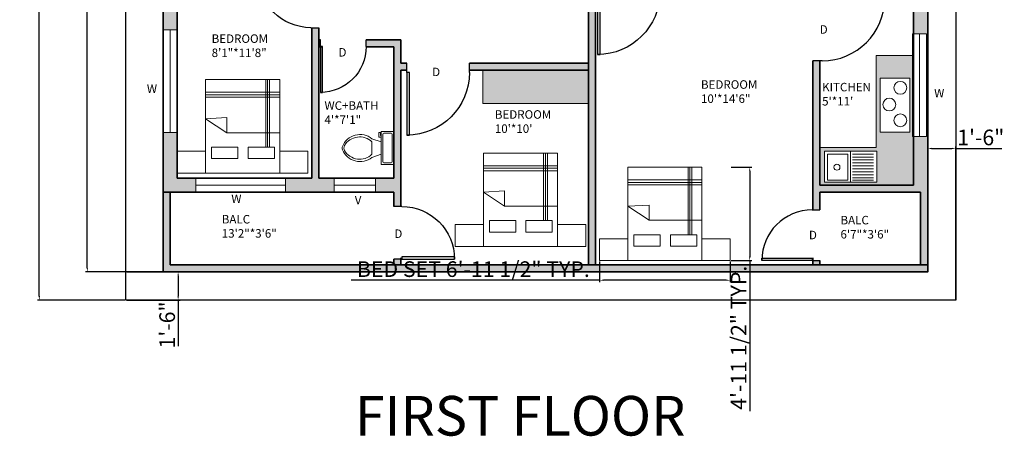
# Model space of a CAD drawing. Units: inches. Extents: x 2048 to 2702, y 2180 to 2964.
# Tile 1 of 3: x 2056 to 2686, y 2180 to 2447. Entities that reach past the tile are written whole.
import ezdxf

# ---------------------------------------------------------------- set-up
doc = ezdxf.new("R2010")
doc.units = ezdxf.units.IN
for name, color, linetype, lineweight in [('A-ANNO-DIMS', 2, 'Continuous', 13), ('A-ANNO-TEXT', 130, 'Continuous', 18), ('A-AREA-IDEN', 130, 'Continuous', 18), ('A-CASE-PATT', 142, 'Continuous', 13), ('A-DOOR', 4, 'Continuous', 25), ('A-EQPM', 142, 'Continuous', 18), ('A-FLOR-FIXT', 142, 'Continuous', 18), ('A-FURN-PATT', 191, 'Continuous', 13), ('A-GLAZ', 4, 'Continuous', 18), ('A-WALL-PATT', 174, 'Continuous', 13), ('bed', 62, 'Continuous', 18), ('C-PROP', 7, 'Continuous', 25), ('kit', 142, 'Continuous', 18), ('TOI', 210, 'Continuous', 18), ('wall', 174, 'Continuous', 35), ('ward', 191, 'Continuous', 18)]:
    doc.layers.add(name, color=color, linetype=linetype, lineweight=lineweight)
doc.styles.get("Standard").update_dxf_attribs({"font": 'arial.ttf'})
doc.dimstyles.new('ISO-25', dxfattribs={"dimtxt": 10, "dimasz": 2.5, "dimexe": 1.25, "dimexo": 0.625, "dimtad": 1, "dimdec": 0, "dimlunit": 4, "dimtxsty": 'Standard', "dimcen": 2.5, "dimadec": 0, "dimazin": 0, "dimtfac": 1, "dimtdec": 0, "dimtmove": 0, "dimatfit": 3, "dimfxl": 1, "dimarcsym": 0})

# ---------------------------------------------------------------- blocks, each defined once
blk = doc.blocks.new('*U2')
for p, q in [((0, 0), (0, -6)), ((40, 0), (40, -6))]:
    blk.add_line(p, q)
blk.add_lwpolyline([(0, 0), (0, 40), (1.75, 40), (1.75, 0)], close=True)
blk.add_arc((0, 0), 40, 0, 90)
blk = doc.blocks.new('*U4')
for p, q in [((9.5, -6), (9.5, -2)), ((-10, -8.5), (-8, -8.5)), ((-10, -9.5), (-10, -8.5)), ((-7, -9.5), (-10, -9.5)), ((-8, -8.5), (-8, -8)), ((-7, -8), (-7, -9.5)), ((-4, -8), (-6, -14)), ((4, -8), (6, -14)), ((4, -14), (-4, -14))]:
    blk.add_line(p, q)
blk.add_lwpolyline([(10.5, -8), (10.5, 0), (-10.5, 0), (-10.5, -8)], close=True)
for points in [[(-9.5, -2), (-9.5, -6)], [(8.5, -1), (-8.5, -1)], [(-8.5, -7), (8.5, -7)]]:
    blk.add_lwpolyline(points)
for centre, radius, start, end in [((-8.62, -1.88), 0.884, 81.8699, 188.1301), ((-8.62, -6.12), 0.884, 171.8699, 278.1301), ((8.62, -1.88), 0.884, 351.8699, 98.1301), ((8.62, -6.12), 0.884, 261.8699, 8.1301), ((3.52, -21.58), 12.17, 141.46911, 247.97143), ((4.2, -21.82), 11.33, 136.36773, 238.94682), ((-3.52, -21.58), 12.17, 292.02843, 38.53071), ((-4.2, -21.82), 11.33, 301.05301, 43.63209), ((0, -27.88), 4, 245.73182, 294.26817), ((0, -29), 4, 254.86053, 285.13947)]:
    blk.add_arc(centre, radius, start, end)
blk = doc.blocks.new('*D11')
at = {"layer": 'A-ANNO-DIMS', "color": 0, "lineweight": -2, "transparency": 16777216}
for p, q in [((2123.4, 2813.51), (2067.51, 2813.51)), ((2068.76, 2270.01), (2068.76, 2811.01)), ((2123.4, 2267.51), (2067.51, 2267.51))]:
    blk.add_line(p, q, dxfattribs=at)
at = {"layer": 'A-ANNO-DIMS', "color": 0, "transparency": 16777216}
for points in [[(2068.35, 2811.01), (2069.18, 2811.01), (2068.76, 2813.51)], [(2068.35, 2270.01), (2069.18, 2270.01), (2068.76, 2267.51)]]:
    blk.add_solid(points, dxfattribs=at)
at = {"layer": 'Defpoints', "color": 0, "transparency": 16777216}
for p in [(2068.76, 2813.51), (2124.03, 2813.51), (2124.03, 2267.51)]:
    blk.add_point(p, dxfattribs=at)
at = {"layer": 'A-ANNO-DIMS', "color": 0, "transparency": 16777216, "insert": (2063.03, 2540.51), "char_height": 10, "attachment_point": 5, "rotation": 90}
blk.add_mtext('45\'-6"', dxfattribs=at)
blk = doc.blocks.new('*D12')
at = {"layer": 'A-ANNO-DIMS', "color": 0, "lineweight": -2, "transparency": 16777216}
for p, q in [((2147.4, 2789.51), (2098.23, 2789.51)), ((2099.48, 2288.01), (2099.48, 2787.01)), ((2147.4, 2285.51), (2098.23, 2285.51))]:
    blk.add_line(p, q, dxfattribs=at)
at = {"layer": 'A-ANNO-DIMS', "color": 0, "transparency": 16777216}
for points in [[(2099.06, 2787.01), (2099.89, 2787.01), (2099.48, 2789.51)], [(2099.06, 2288.01), (2099.89, 2288.01), (2099.48, 2285.51)]]:
    blk.add_solid(points, dxfattribs=at)
at = {"layer": 'Defpoints', "color": 0, "transparency": 16777216}
for p in [(2099.48, 2789.51), (2148.03, 2789.51), (2148.03, 2285.51)]:
    blk.add_point(p, dxfattribs=at)
at = {"layer": 'A-ANNO-DIMS', "color": 0, "transparency": 16777216, "insert": (2093.83, 2537.51), "char_height": 10, "attachment_point": 5, "rotation": 90}
blk.add_mtext("42'", dxfattribs=at)
blk = doc.blocks.new('*D13')
at = {"layer": 'A-ANNO-DIMS', "color": 0, "lineweight": -2, "transparency": 16777216}
for p, q in [((2124.65, 2285.51), (2158.82, 2285.51)), ((2157.57, 2283.01), (2157.57, 2270.01)), ((2124.65, 2267.51), (2158.82, 2267.51)), ((2157.57, 2267.51), (2157.57, 2238.12))]:
    blk.add_line(p, q, dxfattribs=at)
at = {"layer": 'A-ANNO-DIMS', "color": 0, "transparency": 16777216}
for points in [[(2157.15, 2283.01), (2157.99, 2283.01), (2157.57, 2285.51)], [(2157.15, 2270.01), (2157.99, 2270.01), (2157.57, 2267.51)]]:
    blk.add_solid(points, dxfattribs=at)
at = {"layer": 'Defpoints', "color": 0, "transparency": 16777216}
for p in [(2124.03, 2285.51), (2124.03, 2267.51), (2157.57, 2267.51)]:
    blk.add_point(p, dxfattribs=at)
at = {"layer": 'A-ANNO-DIMS', "color": 0, "transparency": 16777216, "insert": (2151.84, 2251.57), "char_height": 10, "attachment_point": 5, "rotation": 90}
blk.add_mtext('1\'-6"', dxfattribs=at)
blk = doc.blocks.new('*D14')
at = {"layer": 'A-ANNO-DIMS', "color": 0, "lineweight": -2, "transparency": 16777216}
for p, q in [((2637.03, 2286.14), (2637.03, 2365.72)), ((2639.53, 2364.47), (2652.53, 2364.47)), ((2655.03, 2268.14), (2655.03, 2365.72)), ((2655.03, 2364.47), (2684.42, 2364.47))]:
    blk.add_line(p, q, dxfattribs=at)
at = {"layer": 'A-ANNO-DIMS', "color": 0, "transparency": 16777216}
for points in [[(2639.53, 2364.89), (2639.53, 2364.05), (2637.03, 2364.47)], [(2652.53, 2364.89), (2652.53, 2364.05), (2655.03, 2364.47)]]:
    blk.add_solid(points, dxfattribs=at)
at = {"layer": 'Defpoints', "color": 0, "transparency": 16777216}
for p in [(2655.03, 2364.47), (2637.03, 2285.51), (2655.03, 2267.51)]:
    blk.add_point(p, dxfattribs=at)
at = {"layer": 'A-ANNO-DIMS', "color": 0, "transparency": 16777216, "insert": (2670.97, 2370.2), "char_height": 10, "attachment_point": 5}
blk.add_mtext('1\'-6"', dxfattribs=at)
blk = doc.blocks.new('BED-DOUBLE-NIGHTSTANDS')
for p, q in [((24.5, 43.17), (24.5, 0)), ((25.71, 43.17), (25.71, 0)), ((26.92, 43.17), (26.92, 0)), ((18.01, 33.96), (51.87, 33.96)), ((51.87, 33.96), (65.5, 24.98)), ((51.87, 24.18), (51.87, 33.96)), ((65.5, 24.98), (51.87, 24.18)), ((18.01, 11.29), (65.5, 11.29)), ((18.01, 9.68), (65.5, 9.68)), ((18.01, 8.07), (65.5, 8.07))]:
    blk.add_line(p, q)
for points in [[(18.01, 59.74), (0, 59.74), (0, 45.7), (18.01, 45.7)], [(18.01, 59.74), (65.5, 59.74), (65.5, 0), (18.01, 0)], [(83.51, 59.74), (65.5, 59.74), (65.5, 45.7), (83.51, 45.7)], [(21.39, 50.51), (38.23, 50.51), (38.23, 43.17), (21.39, 43.17)], [(44.78, 50.51), (61.62, 50.51), (61.62, 43.17), (44.78, 43.17)]]:
    blk.add_lwpolyline(points, close=True)
blk = doc.blocks.new('COOKTOP-3-BURNER')
blk.add_lwpolyline([(0, 0), (34.65, 0), (34.65, 18.99), (0, 18.99)], close=True)
for centre in [(6.24, 12.85), (27.06, 12.85), (16.95, 5.75)]:
    blk.add_circle(centre, 4.1)
blk = doc.blocks.new('SINK-WITH-DRAINER')
for p, q in [((2.08, 18.11), (2.08, 31.52)), ((3.85, 18.11), (3.85, 31.52)), ((5.62, 18.11), (5.62, 31.52)), ((7.59, 18.11), (7.59, 31.52)), ((9.36, 18.11), (9.36, 31.52)), ((11.32, 18.11), (11.32, 31.52)), ((13.22, 18.11), (13.22, 31.52)), ((15.25, 18.11), (15.25, 31.52)), ((17.15, 18.11), (17.15, 31.52)), ((18.67, 18.11), (18.67, 31.52)), ((0, 16.82), (19.98, 16.82))]:
    blk.add_line(p, q)
for points in [[(0, 0), (19.98, 0), (19.98, 33.65), (0, 33.65)], [(1.93, 1.93), (18.53, 1.93), (18.53, 15.13), (1.93, 15.13)]]:
    blk.add_lwpolyline(points, close=True)
blk.add_circle((10.31, 8.05), 1.95)
blk = doc.blocks.new('WINDOW-WIDE')
blk.add_line((0, 4.49), (65.63, 4.49))
blk.add_lwpolyline([(0, 0), (65.63, 0), (65.63, 8.99), (0, 8.99)], close=True)
blk = doc.blocks.new('*D23')
at = {"layer": 'A-ANNO-DIMS', "color": 0, "lineweight": -2, "transparency": 16777216}
for p, q in [((2427.16, 2292.08), (2427.16, 2278.93)), ((2510.67, 2292.08), (2510.67, 2278.93)), ((2427.16, 2280.18), (2268.17, 2280.18)), ((2508.17, 2280.18), (2429.66, 2280.18))]:
    blk.add_line(p, q, dxfattribs=at)
at = {"layer": 'A-ANNO-DIMS', "color": 0, "transparency": 16777216}
for points in [[(2429.66, 2280.6), (2429.66, 2279.77), (2427.16, 2280.18)], [(2508.17, 2280.6), (2508.17, 2279.77), (2510.67, 2280.18)]]:
    blk.add_solid(points, dxfattribs=at)
at = {"layer": 'Defpoints', "color": 0, "transparency": 16777216}
for p in [(2427.16, 2292.71), (2510.67, 2292.71), (2427.16, 2280.18)]:
    blk.add_point(p, dxfattribs=at)
at = {"layer": 'A-ANNO-DIMS', "color": 0, "transparency": 16777216, "insert": (2346.41, 2285.98), "char_height": 10, "attachment_point": 5}
blk.add_mtext('BED SET 6\'-11 1/2" TYP.', dxfattribs=at)
blk = doc.blocks.new('*D24')
at = {"layer": 'A-ANNO-DIMS', "color": 0, "lineweight": -2, "transparency": 16777216}
for p, q in [((2511.3, 2352.45), (2524.45, 2352.45)), ((2523.2, 2349.95), (2523.2, 2295.21)), ((2511.3, 2292.71), (2524.45, 2292.71)), ((2523.2, 2292.71), (2523.2, 2196.53))]:
    blk.add_line(p, q, dxfattribs=at)
at = {"layer": 'A-ANNO-DIMS', "color": 0, "transparency": 16777216}
for points in [[(2522.78, 2349.95), (2523.62, 2349.95), (2523.2, 2352.45)], [(2522.78, 2295.21), (2523.62, 2295.21), (2523.2, 2292.71)]]:
    blk.add_solid(points, dxfattribs=at)
at = {"layer": 'Defpoints', "color": 0, "transparency": 16777216}
for p in [(2510.67, 2352.45), (2510.67, 2292.71), (2523.2, 2292.71)]:
    blk.add_point(p, dxfattribs=at)
at = {"layer": 'A-ANNO-DIMS', "color": 0, "transparency": 16777216, "insert": (2517.4, 2243.37), "char_height": 10, "attachment_point": 5, "rotation": 90}
blk.add_mtext('4\'-11 1/2" TYP.', dxfattribs=at)

msp = doc.modelspace()

# ---------------------------------------------------------------- hatches: boundary and pattern name
at = {"layer": 'A-CASE-PATT'}
h = msp.add_hatch(color=256, dxfattribs=at)
h.dxf.hatch_style = 1
h.paths.add_polyline_path([(2264.28, 2565.56), (2181.03, 2565.56), (2181.03, 2601.56), (2157.03, 2601.56), (2157.03, 2541.56), (2264.28, 2541.56)])
h.paths.add_polyline_path([(2178.6, 2563.49), (2159.62, 2563.49), (2159.62, 2598.14), (2178.6, 2598.14)], flags=16)
h.paths.add_polyline_path([(2161.65, 2571.08, -1), (2169.85, 2571.08, -1)], flags=0)
h.paths.add_polyline_path([(2202.29, 2563.69), (2235.94, 2563.69), (2235.94, 2543.71), (2202.29, 2543.71)], flags=16)
h.paths.add_polyline_path([(2204.22, 2561.75), (2217.42, 2561.75), (2217.42, 2545.16), (2204.22, 2545.16)], flags=0)
h.paths.add_polyline_path([(2168.75, 2581.19, -1), (2176.95, 2581.19, -1)], flags=0)
h.paths.add_polyline_path([(2212.29, 2553.38, -1), (2208.39, 2553.38, -1)], flags=0)
h.paths.add_polyline_path([(2161.65, 2591.9, -1), (2169.85, 2591.9, -1)], flags=0)
h.paths.add_polyline_path([(2249.43, 2537.06), (2157.03, 2537.06), (2157.03, 2481.06), (2181.03, 2481.06), (2181.03, 2513.06), (2249.43, 2513.06)])
h.paths.add_polyline_path([(2178.15, 2520.97), (2178.15, 2486.32), (2159.16, 2486.32), (2159.16, 2520.97)], flags=16)
h.paths.add_polyline_path([(2201.45, 2534.49), (2235.1, 2534.49), (2235.1, 2514.51), (2201.45, 2514.51)], flags=16)
h.paths.add_polyline_path([(2203.38, 2532.56), (2216.58, 2532.56), (2216.58, 2515.96), (2203.38, 2515.96)], flags=0)
h.paths.add_polyline_path([(2169.4, 2514.73, -1), (2161.2, 2514.73, -1)], flags=0)
h.paths.add_polyline_path([(2176.5, 2504.02, -1), (2168.3, 2504.02, -1)], flags=0)
h.paths.add_polyline_path([(2211.45, 2524.18, -1), (2207.55, 2524.18, -1)], flags=0)
h.paths.add_polyline_path([(2169.4, 2493.91, -1), (2161.2, 2493.91, -1)], flags=0)
h.paths.add_polyline_path([(2628.03, 2372.19), (2627.36, 2372.19), (2627.36, 2424), (2604.03, 2424), (2604.03, 2365.01), (2568.03, 2365.01), (2568.03, 2341.01), (2628.03, 2341.01)])
h.paths.add_polyline_path([(2606.7, 2374.82), (2606.7, 2409.47), (2625.69, 2409.47), (2625.69, 2374.82)], flags=16)
h.paths.add_polyline_path([(2604.57, 2362.79), (2604.57, 2342.81), (2570.92, 2342.81), (2570.92, 2362.79)], flags=16)
h.paths.add_polyline_path([(2615.46, 2382.4, -1), (2623.66, 2382.4, -1)], flags=0)
h.paths.add_polyline_path([(2608.36, 2392.51, -1), (2616.56, 2392.51, -1)], flags=0)
h.paths.add_polyline_path([(2586.06, 2360.86), (2586.06, 2344.26), (2572.85, 2344.26), (2572.85, 2360.86)], flags=0)
h.paths.add_polyline_path([(2615.46, 2403.23, -1), (2623.66, 2403.23, -1)], flags=0)
h.paths.add_polyline_path([(2580.92, 2352.48, -1), (2577.03, 2352.48, -1)], flags=0)
h.paths.add_polyline_path([(2517.03, 2780.51), (2435.03, 2780.51), (2435.03, 2702.51), (2459.03, 2702.51), (2459.03, 2756.51), (2517.03, 2756.51)])
h.paths.add_polyline_path([(2468.7, 2777.39), (2503.35, 2777.39), (2503.35, 2758.41), (2468.7, 2758.41)], flags=16)
h.paths.add_polyline_path([(2470.84, 2771.26, -1), (2479.04, 2771.26, -1)], flags=0)
h.paths.add_polyline_path([(2457.12, 2739.8), (2457.12, 2706.16), (2437.14, 2706.16), (2437.14, 2739.8)], flags=16)
h.paths.add_polyline_path([(2489.75, 2764.16, -1), (2481.55, 2764.16, -1)], flags=0)
h.paths.add_polyline_path([(2491.66, 2771.26, -1), (2499.86, 2771.26, -1)], flags=0)
h.paths.add_polyline_path([(2455.67, 2721.29), (2455.67, 2708.09), (2439.07, 2708.09), (2439.07, 2721.29)], flags=0)
h.paths.add_polyline_path([(2449.4, 2714.21, -1), (2445.51, 2714.21, -1)], flags=0)
at = {"layer": 'A-FURN-PATT'}
h = msp.add_hatch(color=256, dxfattribs=at)
h.dxf.hatch_style = 1
h.paths.add_polyline_path([(2205.4, 2476.56), (2157.03, 2476.56), (2157.03, 2457.66), (2205.4, 2457.66)])
h.paths.add_polyline_path([(2420.03, 2414.51), (2352.49, 2414.51), (2352.49, 2393.19), (2420.03, 2393.19)])
at = {"layer": 'A-WALL-PATT'}
h = msp.add_hatch(color=256, dxfattribs=at)
h.dxf.hatch_style = 1
h.paths.add_polyline_path([(2300.03, 2293.61), (2295.53, 2293.61), (2295.53, 2290.01), (2300.03, 2290.01)], flags=17)
h.paths.add_polyline_path([(2637.03, 2290.01), (2632.53, 2290.01), (2568.03, 2290.01), (2424.53, 2290.01), (2424.53, 2289.93), (2420.03, 2290.01), (2295.53, 2290.01), (2152.53, 2290.01), (2152.53, 2336.51), (2148.03, 2336.51), (2148.03, 2285.51), (2637.03, 2285.51)])
h.paths.add_polyline_path([(2424.53, 2465.93), (2420.03, 2466.01), (2420.03, 2290.01), (2424.53, 2289.93)])
h.paths.add_polyline_path([(2420.03, 2419.01), (2343.92, 2419.01), (2343.92, 2414.51), (2420.03, 2414.51)])
h.paths.add_polyline_path([(2637.03, 2522.1), (2628.03, 2522.1), (2628.03, 2508.22), (2637.03, 2508.22)])
h.paths.add_polyline_path([(2263.8, 2606.06), (2157.03, 2606.06), (2157.03, 2601.56), (2263.8, 2601.56)])
h.paths.add_polyline_path([(2259.53, 2626.68), (2255.69, 2626.68, -0.004462), (2255.23, 2626.68), (2255.03, 2626.68), (2255.03, 2606.07), (2259.53, 2606.06)])
h.paths.add_polyline_path([(2259.53, 2654.06), (2255.03, 2654.06), (2255.03, 2652.27), (2255.69, 2652.27), (2259.53, 2652.27)])
h.paths.add_polyline_path([(2310.53, 2606.06), (2306.03, 2606.06), (2306.03, 2518.51), (2310.53, 2518.51)])
h.paths.add_polyline_path([(2306.03, 2606.06), (2303.8, 2606.06), (2303.8, 2601.56), (2306.03, 2601.56)])
h.paths.add_polyline_path([(2306.03, 2541.56), (2157.03, 2541.56), (2157.03, 2537.06), (2306.03, 2537.06)])
h.paths.add_polyline_path([(2435.03, 2698.01), (2430.53, 2698.01), (2430.53, 2658.56), (2430.53, 2658.56), (2430.53, 2654.06), (2430.53, 2584.82), (2435.03, 2584.82)])
h.paths.add_polyline_path([(2430.53, 2658.56), (2353.53, 2658.56), (2353.53, 2654.06), (2430.53, 2654.06)])
h.paths.add_polyline_path([(2438.14, 2608.51), (2435.03, 2608.51), (2435.03, 2604.01), (2438.14, 2604.01)])
h = msp.add_hatch(color=256, dxfattribs=at)
h.dxf.hatch_style = 1
h.paths.add_polyline_path([(2637.03, 2621.67), (2628.03, 2621.67), (2628.03, 2608.51), (2628.03, 2587.75), (2637.03, 2587.75)])
h.paths.add_polyline_path([(2637.03, 2685.57), (2628.03, 2685.57), (2628.03, 2661.01), (2521.53, 2661.01), (2521.53, 2662.58), (2517.03, 2662.58), (2517.03, 2656.51), (2517.03, 2637.24), (2521, 2637.24, -0.005), (2521.53, 2637.24), (2521.53, 2656.51), (2628.03, 2656.51), (2628.03, 2647.99), (2637.03, 2647.99)])
h.paths.add_polyline_path([(2568.03, 2292.85), (2563.53, 2292.85), (2563.53, 2290.01), (2568.03, 2290.01)])
h = msp.add_hatch(color=256, dxfattribs=at)
h.dxf.hatch_style = 1
h.paths.add_polyline_path([(2157.03, 2554.63), (2148.03, 2554.63), (2148.03, 2525.8), (2157.03, 2525.8)])
h.paths.add_polyline_path([(2157.03, 2488.27), (2148.03, 2488.27), (2148.03, 2440.26), (2157.03, 2440.26)])
h.paths.add_polyline_path([(2168.96, 2345.51), (2157.03, 2345.51), (2157.03, 2374.63), (2148.03, 2374.63), (2148.03, 2336.51), (2152.53, 2336.51), (2168.96, 2336.51)])
h.paths.add_polyline_path([(2257.35, 2345.51), (2247.53, 2345.51), (2247.53, 2429.51), (2247.53, 2441.68), (2243.03, 2441.68), (2243.03, 2434.01), (2243.03, 2345.51), (2226.28, 2345.51), (2226.28, 2336.51), (2257.35, 2336.51)])
h.paths.add_polyline_path([(2300.03, 2414.51), (2303.92, 2414.51), (2303.92, 2419.01), (2300.03, 2419.01), (2300.03, 2434.01), (2277.86, 2434.01), (2277.86, 2429.51), (2295.53, 2429.51), (2295.53, 2409.26), (2295.53, 2345.51), (2283.92, 2345.51), (2283.92, 2336.51), (2295.53, 2336.51), (2295.53, 2327.38), (2300.03, 2327.38)])
h.paths.add_polyline_path([(2637.03, 2481.91), (2628.03, 2481.91), (2628.03, 2470.51), (2521.21, 2470.51), (2521.21, 2466.01), (2563.53, 2466.01), (2563.53, 2460.5), (2568.03, 2460.5), (2568.03, 2466.01), (2628.03, 2466.01), (2628.03, 2437.82), (2636.35, 2437.82), (2636.35, 2372.19), (2628.03, 2372.19), (2628.03, 2341.01), (2568.03, 2341.01), (2568.03, 2365.01), (2568.03, 2420.5), (2563.53, 2420.5), (2563.53, 2341.01), (2563.53, 2325.13), (2568.03, 2325.13), (2568.03, 2336.51), (2632.53, 2336.51), (2632.53, 2290.01), (2637.03, 2290.01)])
h.paths.add_polyline_path([(2263.16, 2481.06), (2162.03, 2481.06), (2157.03, 2481.06), (2157.03, 2476.56), (2205.4, 2476.56), (2263.16, 2476.56)])
h.paths.add_polyline_path([(2435.03, 2533.49), (2431.18, 2533.49), (2430.53, 2533.49), (2430.53, 2523.01), (2310.53, 2523.01), (2310.53, 2518.51), (2430.53, 2518.51), (2456.56, 2518.51), (2481.53, 2518.51), (2481.53, 2470.51), (2465.77, 2470.51), (2465.77, 2466.01), (2489.41, 2466.01), (2489.41, 2470.51), (2486.03, 2470.51), (2486.03, 2518.51), (2628.03, 2518.51), (2628.03, 2523.01), (2435.03, 2523.01)])
h.paths.add_polyline_path([(2310.53, 2518.51), (2306.03, 2518.51), (2306.03, 2481.06), (2303.16, 2481.06), (2303.16, 2476.56), (2310.53, 2476.56)])

# ---------------------------------------------------------------- linework, layer by layer
at = {"layer": 'A-GLAZ'}
for p, q in [((2168.96, 2341.01), (2226.28, 2341.01)), ((2257.35, 2341.01), (2283.92, 2341.01))]:
    msp.add_line(p, q, dxfattribs=at)
for points in [[(2168.96, 2336.51), (2226.28, 2336.51), (2226.28, 2345.51), (2168.96, 2345.51)], [(2257.35, 2336.51), (2283.92, 2336.51), (2283.92, 2345.51), (2257.35, 2345.51)]]:
    msp.add_lwpolyline(points, close=True, dxfattribs=at)
at = {"layer": 'C-PROP'}
for p, q in [((2124.03, 2267.51), (2124.03, 2813.51)), ((2655.03, 2813.51), (2655.03, 2267.51)), ((2655.03, 2267.51), (2124.03, 2267.51))]:
    msp.add_line(p, q, dxfattribs=at)
at = {"layer": 'kit'}
for p, q in [((2628.03, 2424), (2604.03, 2424)), ((2604.03, 2424), (2604.03, 2365.01)), ((2568.03, 2341.01), (2568.03, 2365.01)), ((2568.03, 2365.01), (2604.03, 2365.01))]:
    msp.add_line(p, q, dxfattribs=at)
at = {"layer": 'wall'}
for p, q in [((2420.03, 2419.01), (2420.03, 2470.51)), ((2424.53, 2294.51), (2424.53, 2466.01)), ((2243.03, 2434.01), (2243.03, 2441.68)), ((2247.53, 2429.51), (2247.53, 2441.68)), ((2243.03, 2345.51), (2243.03, 2434.01)), ((2247.53, 2434.01), (2248.57, 2434.01)), ((2277.86, 2434.01), (2300.03, 2434.01)), ((2300.03, 2434.01), (2300.03, 2419.01)), ((2247.53, 2345.51), (2247.53, 2429.51)), ((2247.53, 2429.51), (2249.85, 2429.51)), ((2277.86, 2429.51), (2295.53, 2429.51)), ((2295.53, 2429.51), (2295.53, 2409.26)), ((2295.53, 2419.01), (2295.53, 2345.51)), ((2303.92, 2419.01), (2300.03, 2419.01)), ((2420.03, 2419.01), (2343.92, 2419.01)), ((2563.53, 2420.5), (2563.53, 2341.01)), ((2568.03, 2420.5), (2568.03, 2341.01)), ((2300.03, 2414.51), (2300.03, 2327.38)), ((2300.03, 2414.51), (2300.03, 2409.26)), ((2303.92, 2414.51), (2300.03, 2414.51)), ((2420.03, 2414.51), (2343.92, 2414.51)), ((2420.03, 2294.51), (2420.03, 2414.51)), ((2420.03, 2294.51), (2420.03, 2414.51)), ((2157.03, 2345.51), (2243.03, 2345.51)), ((2295.53, 2345.51), (2247.53, 2345.51)), ((2247.53, 2345.51), (2295.53, 2345.51)), ((2563.53, 2341.01), (2563.53, 2325.13)), ((2628.03, 2341.01), (2568.03, 2341.01)), ((2152.53, 2336.51), (2148.03, 2336.51)), ((2152.53, 2336.51), (2295.53, 2336.51)), ((2152.53, 2290.01), (2152.53, 2336.51)), ((2295.53, 2336.51), (2295.53, 2327.38)), ((2632.53, 2336.51), (2568.03, 2336.51)), ((2568.03, 2336.51), (2568.03, 2325.13)), ((2632.53, 2290.01), (2632.53, 2336.51)), ((2148.03, 2285.51), (2148.03, 2305.5)), ((2295.53, 2293.61), (2295.53, 2290.01)), ((2300.03, 2294.51), (2300.03, 2290.01)), ((2420.03, 2294.51), (2420.03, 2290.01)), ((2424.53, 2294.51), (2424.53, 2290.01)), ((2563.53, 2294.51), (2563.53, 2290.01)), ((2568.03, 2292.85), (2568.03, 2290.01)), ((2148.03, 2285.51), (2148.03, 2290.01)), ((2152.53, 2290.01), (2295.53, 2290.01)), ((2295.53, 2290.01), (2420.03, 2290.01)), ((2424.53, 2290.01), (2602.57, 2290.01)), ((2632.53, 2290.01), (2568.03, 2290.01)), ((2632.53, 2290.01), (2637.03, 2290.01)), ((2637.03, 2285.51), (2637.03, 2290.01)), ((2148.03, 2285.51), (2152.53, 2285.51)), ((2637.03, 2285.51), (2628.49, 2285.51)), ((2637.03, 2285.51), (2632.53, 2285.51))]:
    msp.add_line(p, q, dxfattribs=at)
for points in [[(2148.03, 2285.51), (2637.03, 2285.51), (2637.03, 2789.51), (2148.03, 2789.51)], [(2420.03, 2290.01), (2424.53, 2289.93), (2424.53, 2465.93), (2420.03, 2466.01)]]:
    msp.add_lwpolyline(points, close=True, dxfattribs=at)
for points in [[(2628.03, 2661.01), (2628.03, 2780.51), (2157.03, 2780.51), (2157.03, 2345.51)], [(2628.03, 2341.01), (2628.03, 2466.01)]]:
    msp.add_lwpolyline(points, dxfattribs=at)
at = {"layer": 'ward'}
msp.add_lwpolyline([(2352.49, 2414.51), (2420.03, 2414.51), (2420.03, 2393.19), (2352.49, 2393.19)], close=True, dxfattribs=at)

# ---------------------------------------------------------------- block references
at = {"layer": 'A-DOOR'}
for p, xscale, yscale, zscale, rotation in [((2242.5, 2475.2), -0.8377984646543621, 0.8377984646543621, 0.8377984646543621, 90), ((2248.57, 2429.62), -0.7322633769374338, 0.7322633769374338, 0.7322633769374338, 180), ((2300.59, 2293.61), -0.8441697781492633, 0.8441697781492633, 0.8441697781492633, 270), ((2563.18, 2292.85), 0.8070227505798396, 0.8070227505798396, 0.8070227505798396, 90)]:
    msp.add_blockref('*U2', p, dxfattribs=dict(at, xscale=xscale, yscale=yscale, zscale=zscale, rotation=rotation))
at = {"layer": 'A-DOOR', "xscale": -1, "rotation": 180}
for p in [(2425.77, 2464.51), (2303.92, 2413.01)]:
    msp.add_blockref('*U2', p, dxfattribs=at)
at = {"layer": 'A-DOOR', "rotation": 270}
msp.add_blockref('*U2', (2569.53, 2460.5), dxfattribs=at)
at = {"layer": 'A-EQPM', "rotation": 269.9999999999995}
msp.add_blockref('COOKTOP-3-BURNER', (2606.7, 2409.47), dxfattribs=at)
at = {"layer": 'A-FLOR-FIXT', "rotation": 269.9999999999999}
msp.add_blockref('SINK-WITH-DRAINER', (2570.92, 2362.79), dxfattribs=at)
at = {"layer": 'A-GLAZ'}
for p, rotation in [((2148.04, 2440.26), 270), ((2627.36, 2437.82), 269.9999999999994)]:
    msp.add_blockref('WINDOW-WIDE', p, dxfattribs=dict(at, rotation=rotation))
at = {"layer": 'bed', "rotation": 180}
for p in [(2240.54, 2408.45), (2418.3, 2361.48), (2510.67, 2352.45)]:
    msp.add_blockref('BED-DOUBLE-NIGHTSTANDS', p, dxfattribs=at)
at = {"layer": 'TOI', "rotation": 270}
msp.add_blockref('*U4', (2295.53, 2364.71), dxfattribs=at)

# ---------------------------------------------------------------- texts
at = {"layer": 'A-ANNO-TEXT', "attachment_point": 1}
for s, width, gutter_width, heights, insert, char_height in [('D', 134.4203, 27.16, [14.7], (2567.96, 2443.25), 5.43), ('D', 134.4203, 27.16, [14.7], (2260.15, 2428.64), 5.43), ('D', 134.4203, 27.16, [14.7], (2320.04, 2416.12), 5.43), ('W', 134.4203, 27.16, [14.7], (2137.58, 2405.36), 5.43), ('W', 134.4203, 27.16, [14.7], (2641.17, 2402.53), 5.43), ('W', 134.4203, 27.16, [14.7], (2191.59, 2334.99), 5.43), ('V', 134.4203, 27.16, [14.7], (2270.54, 2334.13), 5.43), ('D', 134.4203, 27.16, [14.7], (2295.89, 2312.65), 5.43), ('D', 134.4203, 27.16, [14.7], (2561.07, 2311.81), 5.43), ('FIRST FLOOR', 6945.6286, 126.82, [0], (2270.55, 2206.18), 25.3642)]:
    msp.add_mtext_dynamic_manual_height_columns(s, width=width, gutter_width=gutter_width, heights=heights, dxfattribs=dict(at, insert=insert, char_height=char_height))
at = {"layer": 'A-AREA-IDEN', "char_height": 5.433, "attachment_point": 1}
for s, insert in [('BEDROOM\\P8\'1"*11\'8"', (2179.01, 2437.4)), ('BEDROOM\\P10\'*14\'6"', (2492.01, 2408.06)), ("KITCHEN\\P5'*11'", (2569.5, 2406.42)), ('WC+BATH\\P4\'*7\'1"', (2251.18, 2394.6)), ("BEDROOM\\P10'*10'", (2360.15, 2388.9)), ('BALC\\P13\'2"*3\'6"', (2185.47, 2321.91)), ('BALC\\P6\'7"*3\'6"', (2581.25, 2321.34))]:
    msp.add_mtext_dynamic_manual_height_columns(s, width=134.4203, gutter_width=27.16, heights=[0], dxfattribs=dict(at, insert=insert))

# ---------------------------------------------------------------- dimensions: what is measured, and where the dimension line sits
at = {"layer": 'A-ANNO-DIMS'}
for base, p1, p2, picture, middle in [((2068.76, 2813.51), (2124.03, 2267.51), (2124.03, 2813.51), '*D11', (2063.03, 2540.51)), ((2099.48, 2789.51), (2148.03, 2285.51), (2148.03, 2789.51), '*D12', (2093.83, 2537.51)), ((2157.57, 2267.51), (2124.03, 2285.51), (2124.03, 2267.51), '*D13', (2151.84, 2251.57))]:
    dim = msp.add_linear_dim(base=base, p1=p1, p2=p2, angle=90, dimstyle='ISO-25', override={"dimclrd": 0, "dimclre": 0, "dimclrt": 0}, dxfattribs=at)
    dim.commit()
    dim.dimension.update_dxf_attribs({"geometry": picture, "text_midpoint": middle})
dim = msp.add_linear_dim(base=(2655.03, 2364.47), p1=(2637.03, 2285.51), p2=(2655.03, 2267.51), dimstyle='ISO-25', override={"dimclrd": 0, "dimclre": 0, "dimclrt": 0}, dxfattribs=at)
dim.commit()
dim.dimension.update_dxf_attribs({"geometry": '*D14', "text_midpoint": (2670.97, 2370.2)})
for base, p1, p2, angle, text, picture, middle in [((2523.2, 2292.71), (2510.67, 2352.45), (2510.67, 2292.71), 270, '<> TYP.', '*D24', (2517.4, 2243.37)), ((2427.16, 2280.18), (2510.67, 2292.71), (2427.16, 2292.71), 180, 'BED SET <> TYP.', '*D23', (2346.41, 2285.98))]:
    dim = msp.add_linear_dim(base=base, p1=p1, p2=p2, angle=angle, text=text, dimstyle='ISO-25', override={"dimdec": 1, "dimlfac": 1, "dimrnd": 0, "dimzin": 1, "dimdsep": 46, "dimlunit": 4, "dimfrac": 2}, dxfattribs=at)
    dim.commit()
    dim.dimension.update_dxf_attribs({"geometry": picture, "text_midpoint": middle})

doc.saveas('drawing.dxf')
